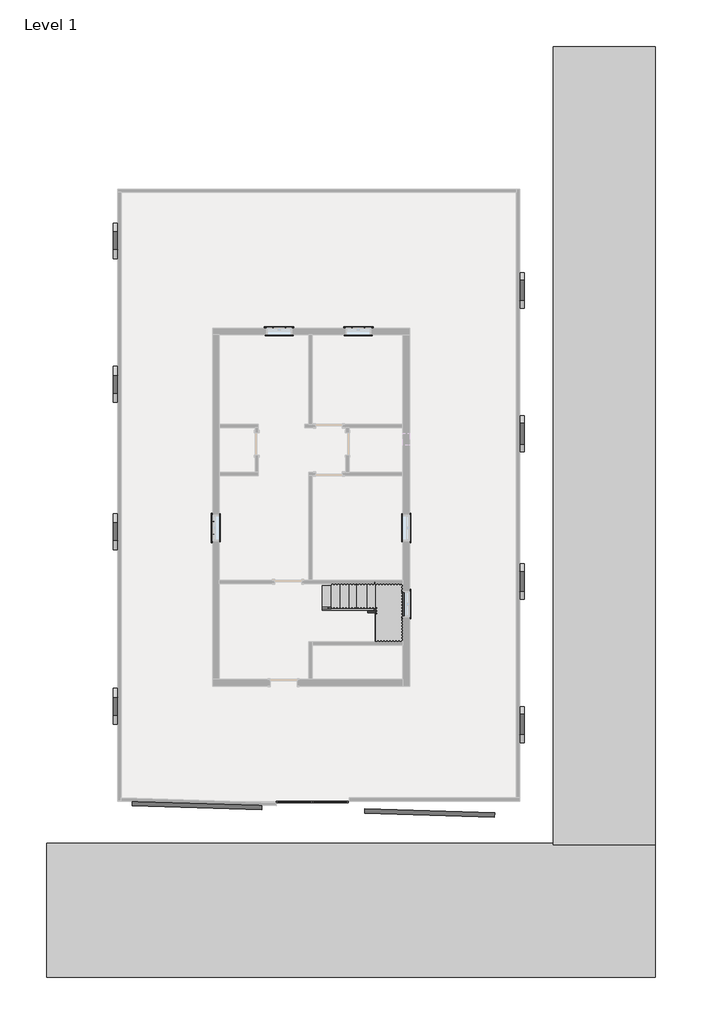
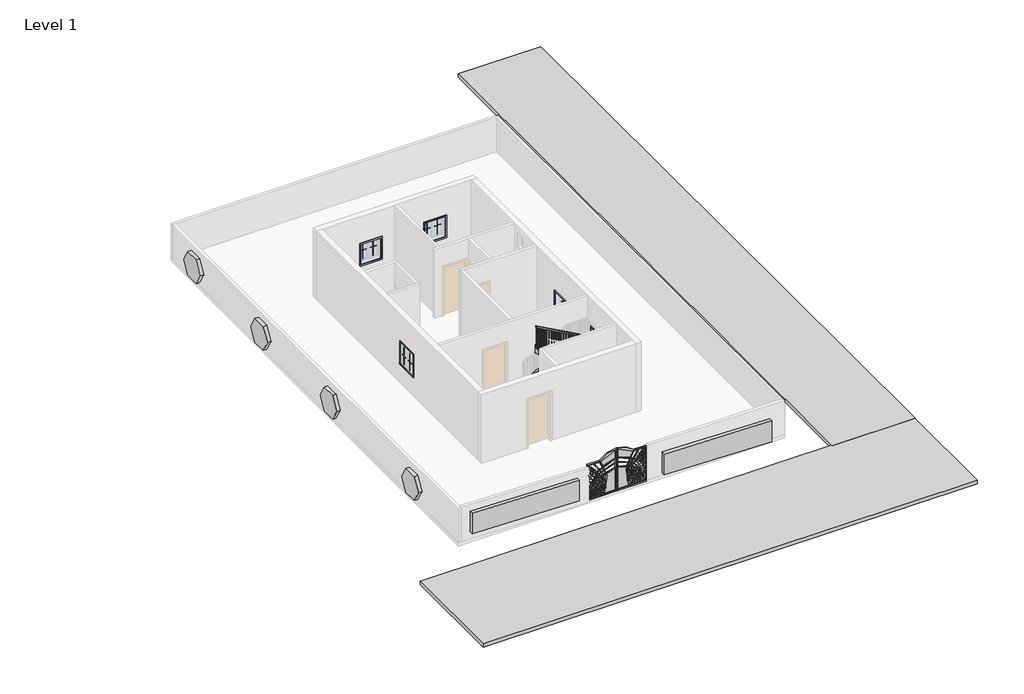
# One storey, part 3 of 3: 25 proxies, 6 members, 1 railing, 1 stair flight.
"""IFC4 building model written with IfcOpenShell, lengths in millimetres."""

from ifc_helpers import new_model, si_unit, frame, origin, place, context, project, spatial, polyline, outline, extrude, faceted_brep, transform, mapped, element, save
from components import generic_models_6bc30956, generic_models_1_generic_models_1_88037803, generic_models_2_generic_models_2_81f0c14a, generic_models_3_generic_models_3_906b0088, generic_models_4_generic_models_4_89f42e2c, muntin_pattern_2x2_muntin_pattern_2x2_b3fe6957, muntin_pattern_2x2_muntin_pattern_2x2_3e0ecaf2, trim_window_exterior_flat_with_sill_41619996, trim_window_interior_flat_picture_frame_51c85655, stair_flight_0b56c5f1

model = new_model("IFC4")

# Units and contexts
model_context = context("Model", 3, world=origin())
ifc_project = project(units=[si_unit("LENGTHUNIT", "METRE", prefix="MILLI")], contexts=[model_context])

# Site, building, storey
site = spatial("IfcSite", under=ifc_project)
building = spatial("IfcBuilding", under=site)
storey = spatial("IfcBuildingStorey", under=building, Name="Level 1", Elevation=0.0)

# Proxies
placement = place(None, origin())
generic_models_shape = generic_models_6bc30956(model_context)
element("IfcBuildingElementProxy", 1, Name="Generic Models", at=placement, inside=storey, context=model_context, shape_type="MappedRepresentation", body=[
    mapped(generic_models_shape, transform((-1222.440747, -9472.0774532, 0.0), x_axis=(1.0, 0.0, 0.0), y_axis=(0.0, 1.0, 0.0), z_axis=(0.0, 0.0, 1.0))),
])
generic_models_1_generic_models_1_shape = generic_models_1_generic_models_1_88037803(model_context)
element("IfcBuildingElementProxy", 2, Name="Generic Models 1 : Generic Models 1", ObjectType="Generic Models 1 : Generic Models 1", at=placement, inside=storey, context=model_context, shape_type="MappedRepresentation", body=[
    mapped(generic_models_1_generic_models_1_shape, transform((0.0, 0.0, 0.0), x_axis=(1.0, 0.0, 0.0), y_axis=(0.0, 1.0, 0.0), z_axis=(0.0, 0.0, 1.0))),
])
generic_models_2_generic_models_2_shape = generic_models_2_generic_models_2_81f0c14a(model_context)
element("IfcBuildingElementProxy", 3, Name="Generic Models 2 : Generic Models 2", ObjectType="Generic Models 2 : Generic Models 2", at=placement, inside=storey, context=model_context, shape_type="MappedRepresentation", body=[
    mapped(generic_models_2_generic_models_2_shape, transform((0.0, 0.0, 0.0), x_axis=(1.0, 0.0, 0.0), y_axis=(0.0, 1.0, 0.0), z_axis=(0.0, 0.0, 1.0))),
])
generic_models_3_generic_models_3_shape = generic_models_3_generic_models_3_906b0088(model_context)
element("IfcBuildingElementProxy", 4, Name="Generic Models 3 : Generic Models 3", ObjectType="Generic Models 3 : Generic Models 3", at=placement, inside=storey, context=model_context, shape_type="MappedRepresentation", body=[
    mapped(generic_models_3_generic_models_3_shape, transform((0.0, 0.0, 0.0), x_axis=(1.0, 0.0, 0.0), y_axis=(0.0, 1.0, 0.0), z_axis=(0.0, 0.0, 1.0))),
])
generic_models_4_generic_models_4_shape = generic_models_4_generic_models_4_89f42e2c(model_context)
element("IfcBuildingElementProxy", 5, Name="Generic Models 4 : Generic Models 4", ObjectType="Generic Models 4 : Generic Models 4", at=placement, inside=storey, context=model_context, shape_type="MappedRepresentation", body=[
    mapped(generic_models_4_generic_models_4_shape, transform((0.0, 0.0, 0.0), x_axis=(1.0, 0.0, 0.0), y_axis=(0.0, 1.0, 0.0), z_axis=(0.0, 0.0, 1.0))),
])
muntin_pattern_2x2_muntin_pattern_2x2_shape = muntin_pattern_2x2_muntin_pattern_2x2_b3fe6957(model_context)
element("IfcBuildingElementProxy", 6, Name="Muntin Pattern_2x2 : Muntin Pattern_2x2", ObjectType="Muntin Pattern_2x2 : Muntin Pattern_2x2", at=placement, inside=storey, context=model_context, shape_type="MappedRepresentation", body=[
    mapped(muntin_pattern_2x2_muntin_pattern_2x2_shape, transform((-2560.703247, 6624.6685985, 984.25), x_axis=(1.0, 0.0, 0.0), y_axis=(0.0, 1.0, 0.0), z_axis=(0.0, 0.0, 1.0))),
])
element("IfcBuildingElementProxy", 7, Name="Muntin Pattern_2x2 : Muntin Pattern_2x2", ObjectType="Muntin Pattern_2x2 : Muntin Pattern_2x2", at=placement, inside=storey, context=model_context, shape_type="MappedRepresentation", body=[
    mapped(muntin_pattern_2x2_muntin_pattern_2x2_shape, transform((134.871753, 6624.6685985, 984.25), x_axis=(1.0, 0.0, 0.0), y_axis=(0.0, 1.0, 0.0), z_axis=(0.0, 0.0, 1.0))),
])
element("IfcBuildingElementProxy", 8, Name="Muntin Pattern_2x2 : Muntin Pattern_2x2", ObjectType="Muntin Pattern_2x2 : Muntin Pattern_2x2", at=placement, inside=storey, context=model_context, shape_type="MappedRepresentation", body=[
    mapped(muntin_pattern_2x2_muntin_pattern_2x2_shape, transform((2082.734253, 41.3060985, 984.25), x_axis=(0.0, -1.0, 0.0), y_axis=(1.0, 0.0, 0.0), z_axis=(0.0, 0.0, 1.0))),
])
element("IfcBuildingElementProxy", 9, Name="Muntin Pattern_2x2 : Muntin Pattern_2x2", ObjectType="Muntin Pattern_2x2 : Muntin Pattern_2x2", at=placement, inside=storey, context=model_context, shape_type="MappedRepresentation", body=[
    mapped(muntin_pattern_2x2_muntin_pattern_2x2_shape, transform((-4603.815747, -387.3189015, 984.25), x_axis=(0.0, 1.0, 0.0), y_axis=(-1.0, 0.0, 0.0), z_axis=(0.0, 0.0, 1.0))),
])
element("IfcBuildingElementProxy", 10, Name="Muntin Pattern_2x2 : Muntin Pattern_2x2", ObjectType="Muntin Pattern_2x2 : Muntin Pattern_2x2", at=placement, inside=storey, context=model_context, shape_type="MappedRepresentation", body=[
    mapped(muntin_pattern_2x2_muntin_pattern_2x2_shape, transform((2082.734253, -2555.8439015, 984.25), x_axis=(0.0, -1.0, 0.0), y_axis=(1.0, 0.0, 0.0), z_axis=(0.0, 0.0, 1.0))),
])
muntin_pattern_2x2_muntin_pattern_2x2_2_shape = muntin_pattern_2x2_muntin_pattern_2x2_3e0ecaf2(model_context)
element("IfcBuildingElementProxy", 11, Name="Muntin Pattern_2x2 : Muntin Pattern_2x2", ObjectType="Muntin Pattern_2x2 : Muntin Pattern_2x2", at=placement, inside=storey, context=model_context, shape_type="MappedRepresentation", body=[
    mapped(muntin_pattern_2x2_muntin_pattern_2x2_2_shape, transform((-2132.078247, 6624.6685985, 984.25), x_axis=(-1.0, 0.0, 0.0), y_axis=(0.0, -1.0, 0.0), z_axis=(0.0, 0.0, 1.0))),
])
element("IfcBuildingElementProxy", 12, Name="Muntin Pattern_2x2 : Muntin Pattern_2x2", ObjectType="Muntin Pattern_2x2 : Muntin Pattern_2x2", at=placement, inside=storey, context=model_context, shape_type="MappedRepresentation", body=[
    mapped(muntin_pattern_2x2_muntin_pattern_2x2_2_shape, transform((563.496753, 6624.6685985, 984.25), x_axis=(-1.0, 0.0, 0.0), y_axis=(0.0, -1.0, 0.0), z_axis=(0.0, 0.0, 1.0))),
])
element("IfcBuildingElementProxy", 13, Name="Muntin Pattern_2x2 : Muntin Pattern_2x2", ObjectType="Muntin Pattern_2x2 : Muntin Pattern_2x2", at=placement, inside=storey, context=model_context, shape_type="MappedRepresentation", body=[
    mapped(muntin_pattern_2x2_muntin_pattern_2x2_2_shape, transform((2082.734253, -387.3189015, 984.25), x_axis=(0.0, 1.0, 0.0), y_axis=(-1.0, 0.0, 0.0), z_axis=(0.0, 0.0, 1.0))),
])
element("IfcBuildingElementProxy", 14, Name="Muntin Pattern_2x2 : Muntin Pattern_2x2", ObjectType="Muntin Pattern_2x2 : Muntin Pattern_2x2", at=placement, inside=storey, context=model_context, shape_type="MappedRepresentation", body=[
    mapped(muntin_pattern_2x2_muntin_pattern_2x2_2_shape, transform((-4603.815747, 41.3060985, 984.25), x_axis=(0.0, -1.0, 0.0), y_axis=(1.0, 0.0, 0.0), z_axis=(0.0, 0.0, 1.0))),
])
element("IfcBuildingElementProxy", 15, Name="Muntin Pattern_2x2 : Muntin Pattern_2x2", ObjectType="Muntin Pattern_2x2 : Muntin Pattern_2x2", at=placement, inside=storey, context=model_context, shape_type="MappedRepresentation", body=[
    mapped(muntin_pattern_2x2_muntin_pattern_2x2_2_shape, transform((2082.734253, -2984.4689015, 984.25), x_axis=(0.0, 1.0, 0.0), y_axis=(-1.0, 0.0, 0.0), z_axis=(0.0, 0.0, 1.0))),
])
trim_window_exterior_flat_with_sill_shape = trim_window_exterior_flat_with_sill_41619996(model_context)
element("IfcBuildingElementProxy", 16, Name="Trim-Window-Exterior-Flat : with Sill", ObjectType="Trim-Window-Exterior-Flat : with Sill", at=placement, inside=storey, context=model_context, shape_type="MappedRepresentation", body=[
    mapped(trim_window_exterior_flat_with_sill_shape, transform((-2346.390747, 6634.1935985, 1828.8), x_axis=(-1.0, 0.0, 0.0), y_axis=(0.0, 0.0, 1.0), z_axis=(0.0, 1.0, 0.0))),
])
element("IfcBuildingElementProxy", 17, Name="Trim-Window-Exterior-Flat : with Sill", ObjectType="Trim-Window-Exterior-Flat : with Sill", at=placement, inside=storey, context=model_context, shape_type="MappedRepresentation", body=[
    mapped(trim_window_exterior_flat_with_sill_shape, transform((349.184253, 6634.1935985, 1828.8), x_axis=(-1.0, 0.0, 0.0), y_axis=(0.0, 0.0, 1.0), z_axis=(0.0, 1.0, 0.0))),
])
element("IfcBuildingElementProxy", 18, Name="Trim-Window-Exterior-Flat : with Sill", ObjectType="Trim-Window-Exterior-Flat : with Sill", at=placement, inside=storey, context=model_context, shape_type="MappedRepresentation", body=[
    mapped(trim_window_exterior_flat_with_sill_shape, transform((2092.259253, -173.0064015, 1828.8), x_axis=(0.0, 1.0, 0.0), y_axis=(0.0, 0.0, 1.0), z_axis=(1.0, 0.0, 0.0))),
])
element("IfcBuildingElementProxy", 19, Name="Trim-Window-Exterior-Flat : with Sill", ObjectType="Trim-Window-Exterior-Flat : with Sill", at=placement, inside=storey, context=model_context, shape_type="MappedRepresentation", body=[
    mapped(trim_window_exterior_flat_with_sill_shape, transform((-4613.340747, -173.0064015, 1828.8), x_axis=(0.0, -1.0, 0.0), y_axis=(0.0, 0.0, 1.0), z_axis=(-1.0, 0.0, 0.0))),
])
element("IfcBuildingElementProxy", 20, Name="Trim-Window-Exterior-Flat : with Sill", ObjectType="Trim-Window-Exterior-Flat : with Sill", at=placement, inside=storey, context=model_context, shape_type="MappedRepresentation", body=[
    mapped(trim_window_exterior_flat_with_sill_shape, transform((2092.259253, -2770.1564015, 1828.8), x_axis=(0.0, 1.0, 0.0), y_axis=(0.0, 0.0, 1.0), z_axis=(1.0, 0.0, 0.0))),
])
trim_window_interior_flat_picture_frame_shape = trim_window_interior_flat_picture_frame_51c85655(model_context)
element("IfcBuildingElementProxy", 21, Name="Trim-Window-Interior-Flat : Picture Frame", ObjectType="Trim-Window-Interior-Flat : Picture Frame", at=placement, inside=storey, context=model_context, shape_type="MappedRepresentation", body=[
    mapped(trim_window_interior_flat_picture_frame_shape, transform((-2346.390747, 6405.5935985, 1828.8), x_axis=(1.0, 0.0, 0.0), y_axis=(0.0, 0.0, 1.0), z_axis=(0.0, -1.0, 0.0))),
])
element("IfcBuildingElementProxy", 22, Name="Trim-Window-Interior-Flat : Picture Frame", ObjectType="Trim-Window-Interior-Flat : Picture Frame", at=placement, inside=storey, context=model_context, shape_type="MappedRepresentation", body=[
    mapped(trim_window_interior_flat_picture_frame_shape, transform((349.184253, 6405.5935985, 1828.8), x_axis=(1.0, 0.0, 0.0), y_axis=(0.0, 0.0, 1.0), z_axis=(0.0, -1.0, 0.0))),
])
element("IfcBuildingElementProxy", 23, Name="Trim-Window-Interior-Flat : Picture Frame", ObjectType="Trim-Window-Interior-Flat : Picture Frame", at=placement, inside=storey, context=model_context, shape_type="MappedRepresentation", body=[
    mapped(trim_window_interior_flat_picture_frame_shape, transform((1863.659253, -173.0064015, 1828.8), x_axis=(0.0, -1.0, 0.0), y_axis=(0.0, 0.0, 1.0), z_axis=(-1.0, 0.0, 0.0))),
])
element("IfcBuildingElementProxy", 24, Name="Trim-Window-Interior-Flat : Picture Frame", ObjectType="Trim-Window-Interior-Flat : Picture Frame", at=placement, inside=storey, context=model_context, shape_type="MappedRepresentation", body=[
    mapped(trim_window_interior_flat_picture_frame_shape, transform((-4384.740747, -173.0064015, 1828.8), x_axis=(0.0, 1.0, 0.0), y_axis=(0.0, 0.0, 1.0), z_axis=(1.0, 0.0, 0.0))),
])
element("IfcBuildingElementProxy", 25, Name="Trim-Window-Interior-Flat : Picture Frame", ObjectType="Trim-Window-Interior-Flat : Picture Frame", at=placement, inside=storey, context=model_context, shape_type="MappedRepresentation", body=[
    mapped(trim_window_interior_flat_picture_frame_shape, transform((1863.659253, -2770.1564015, 1828.8), x_axis=(0.0, -1.0, 0.0), y_axis=(0.0, 0.0, 1.0), z_axis=(-1.0, 0.0, 0.0))),
])

# Members
element("IfcMember", 26, ObjectType="Stringer - 2\" Width", at=placement, inside=storey, context=model_context, shape_type="SweptSolid", body=[
    extrude(outline(polyline([(207.5983948, -879.540747), (0.0, -879.540747), (0.0, -625.5962442), (1261.5333333, 1645.1637558), (1261.5333333, 1017.5421424), (207.5983948, -879.540747)])), frame((0.0, -2065.3064015, 0.0), z_axis=(0.0, 1.0, 0.0), x_axis=(0.0, 0.0, 1.0)), (0.0, 0.0, 1.0), 50.8),
])
element("IfcMember", 27, ObjectType="Stringer - 2\" Width", at=placement, inside=storey, context=model_context, shape_type="SweptSolid", body=[
    extrude(outline(polyline([(1863.659253, -2014.5064015), (1914.459253, -2014.5064015), (1914.459253, -4046.5064015), (1863.659253, -4046.5064015), (1863.659253, -2014.5064015)])), frame((0.0, 0.0, 956.7333333), z_axis=(0.0, 0.0, 1.0), x_axis=(1.0, 0.0, 0.0)), (0.0, 0.0, 1.0), 304.8),
])
element("IfcMember", 28, ObjectType="Stringer - 2\" Width", at=placement, inside=storey, context=model_context, shape_type="SweptSolid", body=[
    extrude(outline(polyline([(956.7333333, 1734.4163636), (2408.9317281, -879.540747), (2060.253054, -879.540747), (956.7333333, 1106.7947502), (956.7333333, 1734.4163636)])), frame((0.0, -4097.3064015, 0.0), z_axis=(0.0, 1.0, 0.0), x_axis=(0.0, 0.0, 1.0)), (0.0, 0.0, 1.0), 50.8),
])
element("IfcMember", 29, ObjectType="Stringer - 2\" Width", at=placement, inside=storey, context=model_context, shape_type="SweptSolid", body=[
    extrude(outline(polyline([(207.5983948, -879.540747), (0.0, -879.540747), (0.0, -625.5962442), (846.6974984, 898.459253), (1195.3761726, 898.459253), (207.5983948, -879.540747)])), frame((0.0, -2979.7064015, 0.0), z_axis=(0.0, 1.0, 0.0), x_axis=(0.0, 0.0, 1.0)), (0.0, 0.0, 1.0), 50.8),
])
element("IfcMember", 30, ObjectType="Stringer - 2\" Width", at=placement, inside=storey, context=model_context, shape_type="SweptSolid", body=[
    extrude(outline(polyline([(898.459253, -2928.9064015), (949.259253, -2928.9064015), (949.259253, -3005.1064015), (898.459253, -3005.1064015), (898.459253, -2928.9064015)])), frame((0.0, 0.0, 956.7333333), z_axis=(0.0, 0.0, 1.0), x_axis=(1.0, 0.0, 0.0)), (0.0, 0.0, 1.0), 304.8),
])
element("IfcMember", 31, ObjectType="Stringer - 2\" Width", at=placement, inside=storey, context=model_context, shape_type="SweptSolid", body=[
    extrude(outline(polyline([(1044.253054, 949.259253), (1392.9317281, 949.259253), (2408.9317281, -879.540747), (2060.253054, -879.540747), (1044.253054, 949.259253)])), frame((0.0, -3055.9064015, 0.0), z_axis=(0.0, 1.0, 0.0), x_axis=(0.0, 0.0, 1.0)), (0.0, 0.0, 1.0), 50.8),
])

# Railing
element("IfcRailing", 32, ObjectType="Handrail - Rectangular", at=placement, inside=storey, context=model_context, shape_type="SolidModel", body=[
    faceted_brep([(-879.540747, -2878.1064015, 1083.7333333), (-879.540747, -2878.1064015, 1025.620221), (-879.540747, -2928.9064015, 1025.620221), (-879.540747, -2928.9064015, 1083.7333333), (873.059253, -2878.1064015, 2057.4), (923.859253, -2878.1064015, 2027.5091099), (923.859253, -2928.9064015, 2027.5091099), (873.059253, -2928.9064015, 2057.4), (873.059253, -2878.1064015, 2099.7333333), (923.859253, -2878.1064015, 2048.9333333), (923.859253, -2928.9064015, 2048.9333333), (873.059253, -2928.9064015, 2099.7333333), (1000.059253, -2878.1064015, 2099.7333333), (1000.059253, -2878.1064015, 2048.9333333), (949.259253, -2928.9064015, 2048.9333333), (949.259253, -2928.9064015, 2099.7333333), (1000.059253, -3005.1064015, 2099.7333333), (1000.059253, -3005.1064015, 2048.9333333), (949.259253, -3005.1064015, 2048.9333333), (949.259253, -3005.1064015, 2099.7333333), (1000.059253, -3055.9064015, 2099.7333333), (949.259253, -3055.9064015, 2099.7333333), (949.259253, -3106.7064015, 2048.9333333), (1000.059253, -3106.7064015, 2048.9333333)], [[[0, 1, 2, 3]], [[1, 0, 4, 5]], [[2, 1, 5, 6]], [[3, 2, 6, 7]], [[0, 3, 7, 4]], [[5, 4, 8, 9]], [[6, 5, 9, 10]], [[7, 6, 10, 11]], [[4, 7, 11, 8]], [[9, 8, 12, 13]], [[10, 9, 13, 14]], [[11, 10, 14, 15]], [[8, 11, 15, 12]], [[13, 12, 16, 17]], [[14, 13, 17, 18]], [[15, 14, 18, 19]], [[12, 15, 19, 16]], [[20, 21, 22, 23]], [[17, 16, 20, 23]], [[18, 17, 23, 22]], [[19, 18, 22, 21]], [[16, 19, 21, 20]]]),
    faceted_brep([(1000.059253, -3055.9064015, 2099.7333333), (1000.059253, -3106.7064015, 2048.9333333), (949.259253, -3106.7064015, 2048.9333333), (949.259253, -3055.9064015, 2099.7333333), (1000.059253, -3055.9064015, 2240.8444444), (949.259253, -3055.9064015, 2210.9535543), (949.259253, -3106.7064015, 2210.9535543), (1000.059253, -3106.7064015, 2240.8444444)], [[[0, 1, 2, 3]], [[4, 5, 6, 7]], [[1, 0, 4, 7]], [[2, 1, 7, 6]], [[3, 2, 6, 5]], [[0, 3, 5, 4]]]),
    faceted_brep([(1000.059253, -3106.7064015, 2240.8444444), (949.259253, -3106.7064015, 2210.9535543), (949.259253, -3055.9064015, 2210.9535543), (1000.059253, -3055.9064015, 2240.8444444), (-879.540747, -3106.7064015, 3285.0666667), (-879.540747, -3055.9064015, 3285.0666667), (-879.540747, -3055.9064015, 3226.9535543), (-879.540747, -3106.7064015, 3226.9535543)], [[[0, 1, 2, 3]], [[4, 5, 6, 7]], [[1, 0, 4, 7]], [[2, 1, 7, 6]], [[3, 2, 6, 5]], [[0, 3, 5, 4]]]),
    extrude(outline(polyline([(3207.5507765, -844.615747), (3218.1341099, -863.665747), (2201.3333333, -863.665747), (2201.3333333, -844.615747), (3207.5507765, -844.615747)])), frame((0.0, -3090.8314015, 0.0), z_axis=(0.0, 1.0, 0.0), x_axis=(0.0, 0.0, 1.0)), (0.0, 0.0, 1.0), 19.05),
    extrude(outline(polyline([(3151.1063321, -743.015747), (3161.6896654, -762.065747), (2201.3333333, -762.065747), (2201.3333333, -743.015747), (3151.1063321, -743.015747)])), frame((0.0, -3090.8314015, 0.0), z_axis=(0.0, 1.0, 0.0), x_axis=(0.0, 0.0, 1.0)), (0.0, 0.0, 1.0), 19.05),
    extrude(outline(polyline([(3094.6618876, -641.415747), (3105.245221, -660.465747), (2201.3333333, -660.465747), (2201.3333333, -641.415747), (3094.6618876, -641.415747)])), frame((0.0, -3090.8314015, 0.0), z_axis=(0.0, 1.0, 0.0), x_axis=(0.0, 0.0, 1.0)), (0.0, 0.0, 1.0), 19.05),
    extrude(outline(polyline([(3038.2174432, -539.815747), (3048.8007765, -558.865747), (2032.0, -558.865747), (2032.0, -539.815747), (3038.2174432, -539.815747)])), frame((0.0, -3090.8314015, 0.0), z_axis=(0.0, 1.0, 0.0), x_axis=(0.0, 0.0, 1.0)), (0.0, 0.0, 1.0), 19.05),
    extrude(outline(polyline([(2981.7729988, -438.215747), (2992.3563321, -457.265747), (2032.0, -457.265747), (2032.0, -438.215747), (2981.7729988, -438.215747)])), frame((0.0, -3090.8314015, 0.0), z_axis=(0.0, 1.0, 0.0), x_axis=(0.0, 0.0, 1.0)), (0.0, 0.0, 1.0), 19.05),
    extrude(outline(polyline([(2925.3285543, -336.615747), (2935.9118876, -355.665747), (2032.0, -355.665747), (2032.0, -336.615747), (2925.3285543, -336.615747)])), frame((0.0, -3090.8314015, 0.0), z_axis=(0.0, 1.0, 0.0), x_axis=(0.0, 0.0, 1.0)), (0.0, 0.0, 1.0), 19.05),
    extrude(outline(polyline([(2868.8841099, -235.015747), (2879.4674432, -254.065747), (1862.6666667, -254.065747), (1862.6666667, -235.015747), (2868.8841099, -235.015747)])), frame((0.0, -3090.8314015, 0.0), z_axis=(0.0, 1.0, 0.0), x_axis=(0.0, 0.0, 1.0)), (0.0, 0.0, 1.0), 19.05),
    extrude(outline(polyline([(2812.4396654, -133.415747), (2823.0229988, -152.465747), (1862.6666667, -152.465747), (1862.6666667, -133.415747), (2812.4396654, -133.415747)])), frame((0.0, -3090.8314015, 0.0), z_axis=(0.0, 1.0, 0.0), x_axis=(0.0, 0.0, 1.0)), (0.0, 0.0, 1.0), 19.05),
    extrude(outline(polyline([(2755.995221, -31.815747), (2766.5785543, -50.865747), (1862.6666667, -50.865747), (1862.6666667, -31.815747), (2755.995221, -31.815747)])), frame((0.0, -3090.8314015, 0.0), z_axis=(0.0, 1.0, 0.0), x_axis=(0.0, 0.0, 1.0)), (0.0, 0.0, 1.0), 19.05),
    extrude(outline(polyline([(2699.5507765, 69.784253), (2710.1341099, 50.734253), (1693.3333333, 50.734253), (1693.3333333, 69.784253), (2699.5507765, 69.784253)])), frame((0.0, -3090.8314015, 0.0), z_axis=(0.0, 1.0, 0.0), x_axis=(0.0, 0.0, 1.0)), (0.0, 0.0, 1.0), 19.05),
    extrude(outline(polyline([(2643.1063321, 171.384253), (2653.6896654, 152.334253), (1693.3333333, 152.334253), (1693.3333333, 171.384253), (2643.1063321, 171.384253)])), frame((0.0, -3090.8314015, 0.0), z_axis=(0.0, 1.0, 0.0), x_axis=(0.0, 0.0, 1.0)), (0.0, 0.0, 1.0), 19.05),
    extrude(outline(polyline([(2586.6618876, 272.984253), (2597.245221, 253.934253), (1693.3333333, 253.934253), (1693.3333333, 272.984253), (2586.6618876, 272.984253)])), frame((0.0, -3090.8314015, 0.0), z_axis=(0.0, 1.0, 0.0), x_axis=(0.0, 0.0, 1.0)), (0.0, 0.0, 1.0), 19.05),
    extrude(outline(polyline([(2530.2174432, 374.584253), (2540.8007765, 355.534253), (1524.0, 355.534253), (1524.0, 374.584253), (2530.2174432, 374.584253)])), frame((0.0, -3090.8314015, 0.0), z_axis=(0.0, 1.0, 0.0), x_axis=(0.0, 0.0, 1.0)), (0.0, 0.0, 1.0), 19.05),
    extrude(outline(polyline([(2473.7729988, 476.184253), (2484.3563321, 457.134253), (1524.0, 457.134253), (1524.0, 476.184253), (2473.7729988, 476.184253)])), frame((0.0, -3090.8314015, 0.0), z_axis=(0.0, 1.0, 0.0), x_axis=(0.0, 0.0, 1.0)), (0.0, 0.0, 1.0), 19.05),
    extrude(outline(polyline([(2417.3285543, 577.784253), (2427.9118876, 558.734253), (1524.0, 558.734253), (1524.0, 577.784253), (2417.3285543, 577.784253)])), frame((0.0, -3090.8314015, 0.0), z_axis=(0.0, 1.0, 0.0), x_axis=(0.0, 0.0, 1.0)), (0.0, 0.0, 1.0), 19.05),
    extrude(outline(polyline([(2360.8841099, 679.384253), (2371.4674432, 660.334253), (1354.6666667, 660.334253), (1354.6666667, 679.384253), (2360.8841099, 679.384253)])), frame((0.0, -3090.8314015, 0.0), z_axis=(0.0, 1.0, 0.0), x_axis=(0.0, 0.0, 1.0)), (0.0, 0.0, 1.0), 19.05),
    extrude(outline(polyline([(2304.4396654, 780.984253), (2315.0229988, 761.934253), (1354.6666667, 761.934253), (1354.6666667, 780.984253), (2304.4396654, 780.984253)])), frame((0.0, -3090.8314015, 0.0), z_axis=(0.0, 1.0, 0.0), x_axis=(0.0, 0.0, 1.0)), (0.0, 0.0, 1.0), 19.05),
    extrude(outline(polyline([(2247.995221, 882.584253), (2258.5785543, 863.534253), (1354.6666667, 863.534253), (1354.6666667, 882.584253), (2247.995221, 882.584253)])), frame((0.0, -3090.8314015, 0.0), z_axis=(0.0, 1.0, 0.0), x_axis=(0.0, 0.0, 1.0)), (0.0, 0.0, 1.0), 19.05),
    extrude(outline(polyline([(965.134253, -2995.5814015), (984.184253, -2995.5814015), (984.184253, -3014.6314015), (965.134253, -3014.6314015), (965.134253, -2995.5814015)])), frame((0.0, 0.0, 1185.3333333), z_axis=(0.0, 0.0, 1.0), x_axis=(1.0, 0.0, 0.0)), (0.0, 0.0, 1.0), 863.6),
    extrude(outline(polyline([(939.734253, -2913.0314015), (939.734253, -2893.9814015), (958.784253, -2893.9814015), (958.784253, -2913.0314015), (939.734253, -2913.0314015)])), frame((0.0, 0.0, 1185.3333333), z_axis=(0.0, 0.0, 1.0), x_axis=(1.0, 0.0, 0.0)), (0.0, 0.0, 1.0), 863.6),
    extrude(outline(polyline([(1990.4674432, 857.184253), (1979.8841099, 838.134253), (1016.0, 838.134253), (1016.0, 857.184253), (1990.4674432, 857.184253)])), frame((0.0, -2913.0314015, 0.0), z_axis=(0.0, 1.0, 0.0), x_axis=(0.0, 0.0, 1.0)), (0.0, 0.0, 1.0), 19.05),
    extrude(outline(polyline([(1934.0229988, 755.584253), (1923.4396654, 736.534253), (1016.0, 736.534253), (1016.0, 755.584253), (1934.0229988, 755.584253)])), frame((0.0, -2913.0314015, 0.0), z_axis=(0.0, 1.0, 0.0), x_axis=(0.0, 0.0, 1.0)), (0.0, 0.0, 1.0), 19.05),
    extrude(outline(polyline([(1877.5785543, 653.984253), (1866.995221, 634.934253), (1016.0, 634.934253), (1016.0, 653.984253), (1877.5785543, 653.984253)])), frame((0.0, -2913.0314015, 0.0), z_axis=(0.0, 1.0, 0.0), x_axis=(0.0, 0.0, 1.0)), (0.0, 0.0, 1.0), 19.05),
    extrude(outline(polyline([(1821.1341099, 552.384253), (1810.5507765, 533.334253), (846.6666667, 533.334253), (846.6666667, 552.384253), (1821.1341099, 552.384253)])), frame((0.0, -2913.0314015, 0.0), z_axis=(0.0, 1.0, 0.0), x_axis=(0.0, 0.0, 1.0)), (0.0, 0.0, 1.0), 19.05),
    extrude(outline(polyline([(1764.6896654, 450.784253), (1754.1063321, 431.734253), (846.6666667, 431.734253), (846.6666667, 450.784253), (1764.6896654, 450.784253)])), frame((0.0, -2913.0314015, 0.0), z_axis=(0.0, 1.0, 0.0), x_axis=(0.0, 0.0, 1.0)), (0.0, 0.0, 1.0), 19.05),
    extrude(outline(polyline([(1708.245221, 349.184253), (1697.6618876, 330.134253), (846.6666667, 330.134253), (846.6666667, 349.184253), (1708.245221, 349.184253)])), frame((0.0, -2913.0314015, 0.0), z_axis=(0.0, 1.0, 0.0), x_axis=(0.0, 0.0, 1.0)), (0.0, 0.0, 1.0), 19.05),
    extrude(outline(polyline([(1651.8007765, 247.584253), (1641.2174432, 228.534253), (677.3333333, 228.534253), (677.3333333, 247.584253), (1651.8007765, 247.584253)])), frame((0.0, -2913.0314015, 0.0), z_axis=(0.0, 1.0, 0.0), x_axis=(0.0, 0.0, 1.0)), (0.0, 0.0, 1.0), 19.05),
    extrude(outline(polyline([(1595.3563321, 145.984253), (1584.7729988, 126.934253), (677.3333333, 126.934253), (677.3333333, 145.984253), (1595.3563321, 145.984253)])), frame((0.0, -2913.0314015, 0.0), z_axis=(0.0, 1.0, 0.0), x_axis=(0.0, 0.0, 1.0)), (0.0, 0.0, 1.0), 19.05),
    extrude(outline(polyline([(1538.9118876, 44.384253), (1528.3285543, 25.334253), (677.3333333, 25.334253), (677.3333333, 44.384253), (1538.9118876, 44.384253)])), frame((0.0, -2913.0314015, 0.0), z_axis=(0.0, 1.0, 0.0), x_axis=(0.0, 0.0, 1.0)), (0.0, 0.0, 1.0), 19.05),
    extrude(outline(polyline([(1482.4674432, -57.215747), (1471.8841099, -76.265747), (508.0, -76.265747), (508.0, -57.215747), (1482.4674432, -57.215747)])), frame((0.0, -2913.0314015, 0.0), z_axis=(0.0, 1.0, 0.0), x_axis=(0.0, 0.0, 1.0)), (0.0, 0.0, 1.0), 19.05),
    extrude(outline(polyline([(1426.0229988, -158.815747), (1415.4396654, -177.865747), (508.0, -177.865747), (508.0, -158.815747), (1426.0229988, -158.815747)])), frame((0.0, -2913.0314015, 0.0), z_axis=(0.0, 1.0, 0.0), x_axis=(0.0, 0.0, 1.0)), (0.0, 0.0, 1.0), 19.05),
    extrude(outline(polyline([(1369.5785543, -260.415747), (1358.995221, -279.465747), (508.0, -279.465747), (508.0, -260.415747), (1369.5785543, -260.415747)])), frame((0.0, -2913.0314015, 0.0), z_axis=(0.0, 1.0, 0.0), x_axis=(0.0, 0.0, 1.0)), (0.0, 0.0, 1.0), 19.05),
    extrude(outline(polyline([(1313.1341099, -362.015747), (1302.5507765, -381.065747), (338.6666667, -381.065747), (338.6666667, -362.015747), (1313.1341099, -362.015747)])), frame((0.0, -2913.0314015, 0.0), z_axis=(0.0, 1.0, 0.0), x_axis=(0.0, 0.0, 1.0)), (0.0, 0.0, 1.0), 19.05),
    extrude(outline(polyline([(1256.6896654, -463.615747), (1246.1063321, -482.665747), (338.6666667, -482.665747), (338.6666667, -463.615747), (1256.6896654, -463.615747)])), frame((0.0, -2913.0314015, 0.0), z_axis=(0.0, 1.0, 0.0), x_axis=(0.0, 0.0, 1.0)), (0.0, 0.0, 1.0), 19.05),
    extrude(outline(polyline([(1200.245221, -565.215747), (1189.6618876, -584.265747), (338.6666667, -584.265747), (338.6666667, -565.215747), (1200.245221, -565.215747)])), frame((0.0, -2913.0314015, 0.0), z_axis=(0.0, 1.0, 0.0), x_axis=(0.0, 0.0, 1.0)), (0.0, 0.0, 1.0), 19.05),
    extrude(outline(polyline([(1143.8007765, -666.815747), (1133.2174432, -685.865747), (169.3333333, -685.865747), (169.3333333, -666.815747), (1143.8007765, -666.815747)])), frame((0.0, -2913.0314015, 0.0), z_axis=(0.0, 1.0, 0.0), x_axis=(0.0, 0.0, 1.0)), (0.0, 0.0, 1.0), 19.05),
    extrude(outline(polyline([(1087.3563321, -768.415747), (1076.7729988, -787.465747), (169.3333333, -787.465747), (169.3333333, -768.415747), (1087.3563321, -768.415747)])), frame((0.0, -2913.0314015, 0.0), z_axis=(0.0, 1.0, 0.0), x_axis=(0.0, 0.0, 1.0)), (0.0, 0.0, 1.0), 19.05),
    extrude(outline(polyline([(965.134253, -3071.7814015), (984.184253, -3071.7814015), (984.184253, -3090.8314015), (965.134253, -3090.8314015), (965.134253, -3071.7814015)])), frame((0.0, 0.0, 1185.3333333), z_axis=(0.0, 0.0, 1.0), x_axis=(1.0, 0.0, 0.0)), (0.0, 0.0, 1.0), 863.6),
    extrude(outline(polyline([(965.134253, -2913.0314015), (965.134253, -2893.9814015), (984.184253, -2893.9814015), (984.184253, -2913.0314015), (965.134253, -2913.0314015)])), frame((0.0, 0.0, 1185.3333333), z_axis=(0.0, 0.0, 1.0), x_axis=(1.0, 0.0, 0.0)), (0.0, 0.0, 1.0), 863.6),
    extrude(outline(polyline([(3216.370221, -860.490747), (3226.9535543, -879.540747), (2201.3333333, -879.540747), (2201.3333333, -860.490747), (3216.370221, -860.490747)])), frame((0.0, -3090.8314015, 0.0), z_axis=(0.0, 1.0, 0.0), x_axis=(0.0, 0.0, 1.0)), (0.0, 0.0, 1.0), 19.05),
    extrude(outline(polyline([(1036.2035543, -860.490747), (1025.620221, -879.540747), (169.3333333, -879.540747), (169.3333333, -860.490747), (1036.2035543, -860.490747)])), frame((0.0, -2913.0314015, 0.0), z_axis=(0.0, 1.0, 0.0), x_axis=(0.0, 0.0, 1.0)), (0.0, 0.0, 1.0), 19.05),
])

# Stair flight
stair_flight_shape = stair_flight_0b56c5f1(model_context)
element("IfcStairFlight", 33, ObjectType="2\" Tread 1\" Nosing 1/4\" Riser", at=placement, inside=storey, context=model_context, shape_type="MappedRepresentation", body=[
    mapped(stair_flight_shape, transform((0.0, 0.0, 0.0), x_axis=(1.0, 0.0, 0.0), y_axis=(0.0, 1.0, 0.0), z_axis=(0.0, 0.0, 1.0))),
])

save(model, "model.ifc")

# Revit data of these elements
# Type
#   m.s. sheet = none
#   2" x2" pipe = none
#   1"x1"pipe = none
#   Default Elevation = 0
# Type "Muntin Pattern_2x2 : Muntin Pattern_2x2"
#   Width [instance default] = 4' - 0"
#   Thickness = 0' - 0 1/2"
#   Height [instance default] = 4' - 0"
#   Distance = 0' - 0 3/4"
#   Interior Material [instance default] = none
#   Exterior Material [instance default] = none
#   Default Elevation = 0
# Type "Trim-Window-Exterior-Flat : with Sill"
#   Trim Width = 0' - 2 1/4"
#   Trim Thickness_Picture Frame = 0' - 1 1/4"
#   Trim Thickness_with Sill = 0' - 0 3/4"
#   Sill Thickness = 0' - 1 1/4"
#   Opening Width [instance default] = 2' - 0"
#   Opening Height [instance default] = 3' - 0"
#   Default Elevation = 4' - 0"
#   Sill = yes
#   Picture Frame = no
#   Trim Material [instance default] = none
# Type "Trim-Window-Interior-Flat : Picture Frame"
#   Trim Thickness_Picture Frame = 0' - 1 1/4"
#   Trim Width = 0' - 2 1/4"
#   Trim Thickness_with Sill = 0' - 0 3/4"
#   Sill Thickness = 0' - 1 1/4"
#   Opening Width [instance default] = 2' - 0"
#   Opening Height [instance default] = 3' - 0"
#   Default Elevation = 4' - 0"
#   Sill = no
#   Picture Frame = yes
#   Trim Material [instance default] = none
# Type "Handrail - Rectangular"
#   Assembly Code = "C2010400"
#   built-in parameter 1008612 = 0.0416667 (stored number, unit not read)
#   built-in parameter 1008611 = 0.0416667 (stored number, unit not read)
#   built-in parameter 1008609 = 0.333333 (stored number, unit not read)
#   built-in parameter 1008604 = 0.166667 (stored number, unit not read)
#   built-in parameter 1008603 = 0.166667 (stored number, unit not read)
#   Railing Height = 3' - 0"
#   built-in parameter 1008630 = 2
#   built-in parameter 1008610 = 2
#   built-in parameter 1008618 = Baluster - Square : 3/4"
# Element 1 (IfcBuildingElementProxy)
#   Phase Created = New Construction
#   Materials on its faces: "r1"
# Element 2 (IfcBuildingElementProxy, "Generic Models 1 : Generic Models 1")
#   Phase Created = New Construction
#   Materials on its faces: "Default Mass Exterior Wall"
# Element 3 (IfcBuildingElementProxy, "Generic Models 2 : Generic Models 2")
#   Phase Created = New Construction
# Element 4 (IfcBuildingElementProxy, "Generic Models 3 : Generic Models 3")
#   Phase Created = New Construction
#   Materials on its faces: "Door - Frame"
# Element 5 (IfcBuildingElementProxy, "Generic Models 4 : Generic Models 4")
#   Phase Created = New Construction
#   Materials on its faces: "Door - Frame"
# Elements 6, 7, 8, 9, 10, 11, 12, 13, 14, 15 (IfcBuildingElementProxy, "Muntin Pattern_2x2 : Muntin Pattern_2x2")
#   Width = 0' - 11 5/8"
#   Height = 2' - 6 1/2"
#   Interior Material = Wood - Stained
#   Exterior Material = Clad - White
#   Phase Created = New Construction
#   Materials on its faces: "Clad - White", "Wood - Stained"
# Elements 16, 17, 18, 19, 20 (IfcBuildingElementProxy, "Trim-Window-Exterior-Flat : with Sill")
#   Opening Width = 2' - 10"
#   Opening Height = 3' - 0"
#   Trim Material = Clad - White
#   Phase Created = New Construction
#   Materials on its faces: "Clad - White"
# Elements 21, 22, 23, 24, 25 (IfcBuildingElementProxy, "Trim-Window-Interior-Flat : Picture Frame")
#   Opening Width = 2' - 10"
#   Opening Height = 3' - 0"
#   Trim Material = Wood - Stained
#   Phase Created = New Construction
#   Materials on its faces: "Wood - Stained"
# Elements 26, 27, 28, 29, 30, 31 (IfcMember, "Stringer - 2\" Width")
#   Phase Created = New Construction
# Element 32 (IfcRailing, "Handrail - Rectangular")
#   Phase Created = New Construction
# Element 33 (IfcStairFlight, "2\" Tread 1\" Nosing 1/4\" Riser")
#   Phase Created = New Construction
# Materials
#   "r1": class "Generic", colour RGB 120 120 120, transparency 0, Cost = 0
#   "Default Mass Exterior Wall": class "Generic", colour RGB 133 178 44, transparency 0.2, Cost = 0
#   "Door - Frame": colour RGB 118 70 51, transparency 0, Cost = 0
#   "Clad - White": class "Wood", colour RGB 242 242 238, transparency 0, Cost = 0
#   "Wood - Stained": class "Wood", colour RGB 224 178 126, transparency 0, Cost = 0
